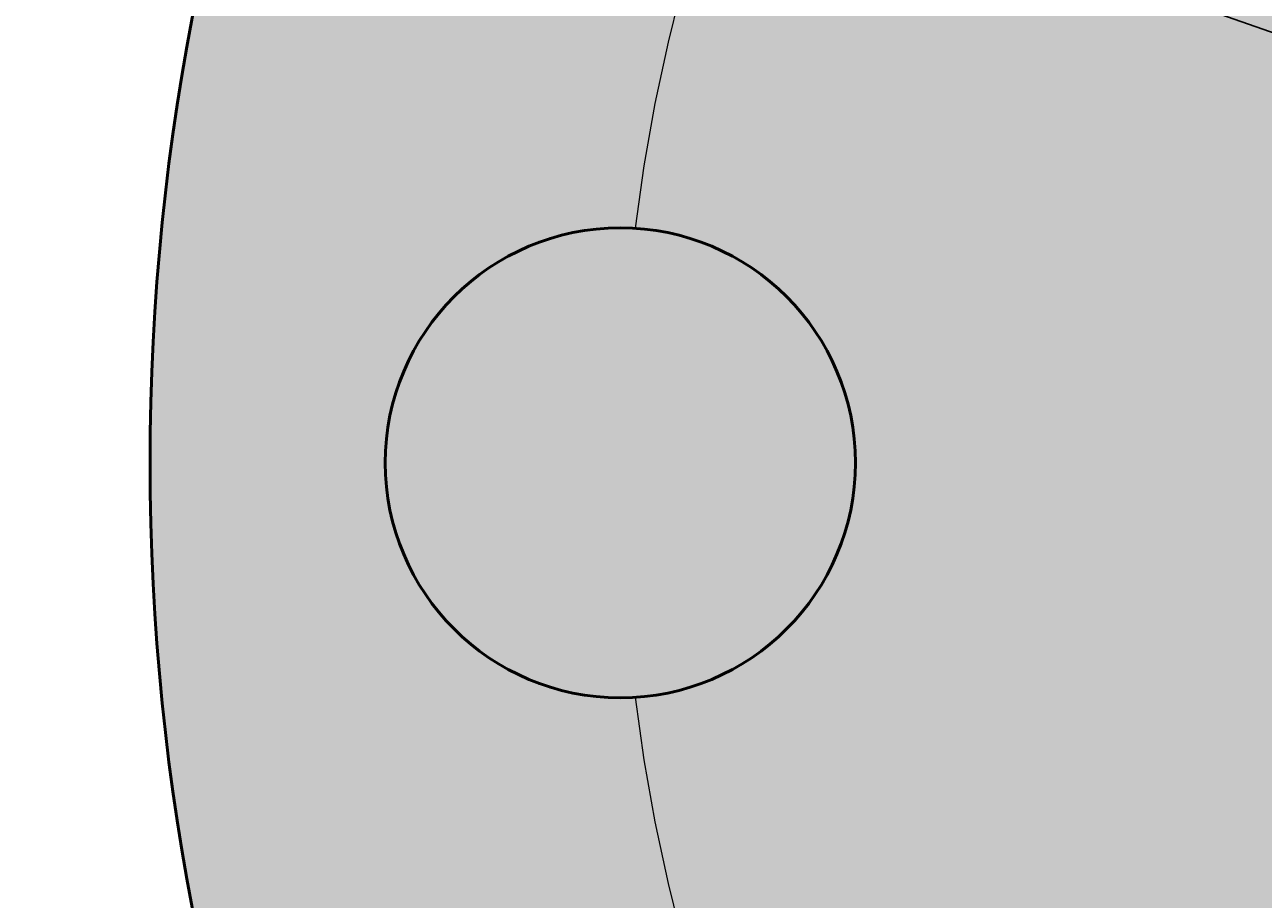
# Model space of a CAD drawing. Units: inches. Extents: x 139261 to 139415, y 52839 to 52963.
# Tile 4 of 20: x 139288 to 139314, y 52891 to 52910. Entities that reach past the tile are written whole.
import ezdxf

# ---------------------------------------------------------------- set-up
doc = ezdxf.new("R2010")
doc.units = ezdxf.units.IN
doc.header["$MEASUREMENT"] = 0
doc.linetypes.add('CENTER', pattern=[50.8, 31.75, -6.35, 6.35, -6.35])
for name, color, linetype, lineweight in [('M-CNTR', 4, 'CENTER', 18), ('M-DIMS', 2, 'Continuous', 25), ('M-HATC', 8, 'Continuous', 18), ('M-OUTL', 7, 'Continuous', 50)]:
    doc.layers.add(name, color=color, linetype=linetype, lineweight=lineweight)
doc.styles.get("Standard").update_dxf_attribs({"font": 'arial.ttf'})
doc.dimstyles.get("Standard").update_dxf_attribs({"dimtxt": 0.18, "dimasz": 0.18, "dimexe": 0.18, "dimexo": 0.0625, "dimgap": 0.09, "dimtad": 0, "dimtih": 1, "dimtoh": 1, "dimdec": 4, "dimzin": 0, "dimdsep": 46, "dimtxsty": 'Standard', "dimcen": 0.09, "dimadec": 0, "dimazin": 0, "dimtfac": 1, "dimtdec": 4, "dimtofl": 0, "dimtmove": 0, "dimatfit": 3, "dimfxl": 1, "dimtolj": 1, "dimtzin": 0, "dimarcsym": 0})

# ---------------------------------------------------------------- blocks, each defined once
blk = doc.blocks.new('*U1')
blk.add_circle((0, 0), 5)
blk = doc.blocks.new('*U2')
at = {"layer": 'M-OUTL', "color": 0, "linetype": 'ByBlock', "lineweight": -2, "transparency": 16777216, "rotation": 90}
blk.add_blockref('*U1', (139300.357, 52900.217), dxfattribs=at)
blk = doc.blocks.new('*D4')
at = {"layer": 'Defpoints', "color": 0, "transparency": 16777216}
for p in [(139373.053, 52923.26), (139307.661, 52877.175)]:
    blk.add_point(p, dxfattribs=at)
at = {"layer": 'M-DIMS', "color": 0, "lineweight": -2, "transparency": 16777216}
for p, q in [((139414.011, 52952.126), (139373.2, 52923.364)), ((139414.191, 52952.126), (139414.011, 52952.126)), ((139340.267, 52900.217), (139340.447, 52900.217)), ((139340.357, 52900.127), (139340.357, 52900.307))]:
    blk.add_line(p, q, dxfattribs=at)
blk.add_arc((139340.357, 52900.217), 40, 34.9168, 52.0771, dxfattribs=at)
at = {"layer": 'M-DIMS', "color": 0, "transparency": 16777216}
blk.add_solid([(139373.183, 52923.388), (139373.217, 52923.339), (139373.053, 52923.26)], dxfattribs=at)
at = {"layer": 'M-DIMS', "color": 0, "transparency": 16777216, "insert": (139414.822, 52952.126), "char_height": 0.18, "attachment_point": 5}
blk.add_mtext('\\A1;∅80.0000', dxfattribs=at)
blk = doc.blocks.new('*D5')
at = {"layer": 'Defpoints', "color": 0, "transparency": 16777216}
for p in [(139316.763, 52908.484), (139363.951, 52891.951)]:
    blk.add_point(p, dxfattribs=at)
at = {"layer": 'M-DIMS', "color": 0, "lineweight": -2, "transparency": 16777216}
for p, q in [((139262.553, 52927.414), (139262.733, 52927.414)), ((139262.733, 52927.414), (139316.593, 52908.544)), ((139340.267, 52900.217), (139340.447, 52900.217)), ((139340.357, 52900.127), (139340.357, 52900.307))]:
    blk.add_line(p, q, dxfattribs=at)
at = {"layer": 'M-DIMS', "color": 0, "transparency": 16777216}
blk.add_solid([(139316.603, 52908.572), (139316.583, 52908.515), (139316.763, 52908.484)], dxfattribs=at)
at = {"layer": 'M-DIMS', "color": 0, "transparency": 16777216, "insert": (139261.922, 52927.414), "char_height": 0.18, "attachment_point": 5}
blk.add_mtext('\\A1;∅50.0000', dxfattribs=at)
blk = doc.blocks.new('*D9')
at = {"layer": 'Defpoints', "color": 0, "transparency": 16777216}
for p in [(139302.054, 52932.357), (139378.659, 52868.078)]:
    blk.add_point(p, dxfattribs=at)
at = {"layer": 'M-DIMS', "color": 0, "lineweight": -2, "transparency": 16777216}
for p, q in [((139278.893, 52951.64), (139279.073, 52951.64)), ((139279.073, 52951.64), (139301.916, 52932.472)), ((139340.267, 52900.217), (139340.447, 52900.217)), ((139340.357, 52900.127), (139340.357, 52900.307))]:
    blk.add_line(p, q, dxfattribs=at)
at = {"layer": 'M-DIMS', "color": 0, "transparency": 16777216}
blk.add_solid([(139301.936, 52932.495), (139301.897, 52932.449), (139302.054, 52932.357)], dxfattribs=at)
at = {"layer": 'M-DIMS', "color": 0, "transparency": 16777216, "insert": (139278.506, 52951.64), "char_height": 0.18, "attachment_point": 5}
blk.add_mtext('\\A1;∅100', dxfattribs=at)

msp = doc.modelspace()

# ---------------------------------------------------------------- hatches: boundary and pattern name
at = {"layer": 'M-HATC'}
h = msp.add_hatch(color=256, dxfattribs=at)
h.dxf.hatch_style = 1
h.paths.add_polyline_path([(139290.35689, 52900.21749, 1), (139390.35689, 52900.21749, 1)])
h.paths.add_polyline_path([(139335.36666, 52939.90499, -0.01563646), (139335.35689, 52940.21749, -1), (139345.35689, 52940.21749, -0.01563646), (139345.34711, 52939.90499, -0.13461315), (139364.89157, 52931.80941, -0.691035), (139373.64116, 52928.50176, -0.21521822), (139371.94881, 52924.75216, -0.13461315), (139380.04439, 52905.20771, -0.43265224), (139385.35689, 52900.21749, -0.43265224), (139380.04439, 52895.22726, -0.13461315), (139371.94881, 52875.68281, -0.21521822), (139373.64116, 52871.93321, -0.691035), (139364.89157, 52868.62556, -0.13461315), (139345.34711, 52860.52999, -0.01563646), (139345.35689, 52860.21749, -1), (139335.35689, 52860.21749, -0.01563646), (139335.36666, 52860.52999, -0.13461315), (139315.82221, 52868.62556, -0.691035), (139307.07262, 52871.93321, -0.21521822), (139308.76496, 52875.68281, -0.13461315), (139300.66939, 52895.22726, -0.43265224), (139295.35689, 52900.21749, -0.43265224), (139300.66939, 52905.20771, -0.13461315), (139308.76496, 52924.75216, -0.21521822), (139307.07262, 52928.50176, -0.691035), (139315.82221, 52931.80941, -0.13461315)], flags=16)
h.paths.add_polyline_path([(139365.35689, 52900.21749, -1), (139315.35689, 52900.21749, -1)], flags=0)
h.paths.add_polyline_path([(139323.71474, 52911.30978), (139356.99903, 52911.30978, -0.3027197), (139356.99903, 52889.12519), (139323.71474, 52889.12519, -0.3027197)], flags=0)
h.paths.add_polyline_path([(139364.89157, 52931.80941, 0.13461315), (139345.34711, 52939.90499, -0.93933644), (139335.36666, 52939.90499, 0.13461315), (139315.82221, 52931.80941, -0.18270763), (139317.07262, 52928.50176, -0.64579494), (139308.76496, 52924.75216, 0.13461315), (139300.66939, 52905.20771, -0.39601219), (139305.35689, 52900.21749, -0.39601219), (139300.66939, 52895.22726, 0.13461315), (139308.76496, 52875.68281, -0.64579494), (139317.07262, 52871.93321, -0.18270763), (139315.82221, 52868.62556, 0.13461315), (139335.36666, 52860.52999, -0.93933644), (139345.34711, 52860.52999, 0.13461315), (139364.89157, 52868.62556, -0.18270763), (139363.64116, 52871.93321, -0.64579494), (139371.94881, 52875.68281, 0.13461315), (139380.04439, 52895.22726, -0.39601219), (139375.35689, 52900.21749, -0.39601219), (139380.04439, 52905.20771, 0.13461315), (139371.94881, 52924.75216, -0.64579494), (139363.64116, 52928.50176, -0.18270763)], flags=0)
h = msp.add_hatch(color=256, dxfattribs=at)
h.dxf.hatch_style = 1
h.set_gradient(color1=(205, 105, 40), tint=1)
h.paths.add_polyline_path([(139335.35689, 52940.21749, 1), (139345.35689, 52940.21749, 1)])
h.paths.add_polyline_path([(139307.07262, 52928.50176, 1), (139317.07262, 52928.50176, 1)])
h.paths.add_polyline_path([(139295.35689, 52900.21749, 1), (139305.35689, 52900.21749, 1)])
h.paths.add_polyline_path([(139307.07262, 52871.93321, 1), (139317.07262, 52871.93321, 1)])
h.paths.add_polyline_path([(139345.35689, 52860.21749, 1), (139335.35689, 52860.21749, 1)])
h.paths.add_polyline_path([(139363.64116, 52871.93321, 1), (139373.64116, 52871.93321, 1)])
h.paths.add_polyline_path([(139375.35689, 52900.21749, 1), (139385.35689, 52900.21749, 1)])
h.paths.add_polyline_path([(139363.64116, 52928.50176, 1), (139373.64116, 52928.50176, 1)])
h = msp.add_hatch(color=256, dxfattribs=at)
h.dxf.hatch_style = 1
h.paths.add_polyline_path([(139345.34711, 52939.90499, -0.93933644), (139335.36666, 52939.90499, 0.13461315), (139315.82221, 52931.80941, -0.18270763), (139317.07262, 52928.50176, -0.64579494), (139308.76496, 52924.75216, 0.13461315), (139300.66939, 52905.20771, -0.39601219), (139305.35689, 52900.21749, -0.39601219), (139300.66939, 52895.22726, 0.13461315), (139308.76496, 52875.68281, -0.64579494), (139317.07262, 52871.93321, -0.18270763), (139315.82221, 52868.62556, 0.13461315), (139335.36666, 52860.52999, -0.93933644), (139345.34711, 52860.52999, 0.13461315), (139364.89157, 52868.62556, -0.18270763), (139363.64116, 52871.93321, -0.64579494), (139371.94881, 52875.68281, 0.13461315), (139380.04439, 52895.22726, -0.39601219), (139375.35689, 52900.21749, -0.39601219), (139380.04439, 52905.20771, 0.13461315), (139371.94881, 52924.75216, -0.64579494), (139363.64116, 52928.50176, -0.18270763), (139364.89157, 52931.80941, 0.13461315)])
h.paths.add_polyline_path([(139365.35689, 52900.21749, -1), (139315.35689, 52900.21749, -1)], flags=16)
h.paths.add_polyline_path([(139356.99903, 52911.30978, -0.3027197), (139356.99903, 52889.12519), (139323.71474, 52889.12519, -0.3027197), (139323.71474, 52911.30978)], flags=0)

# ---------------------------------------------------------------- linework, layer by layer
at = {"layer": 'M-CNTR'}
for start, end in [(142.166643, 172.833357), (187.166643, 217.833357)]:
    msp.add_arc((139340.35689, 52900.21749), 40, start, end, dxfattribs=at)
at = {"layer": 'M-OUTL'}
msp.add_circle((139340.35689, 52900.21749), 50, dxfattribs=at)

# ---------------------------------------------------------------- block references
msp.add_blockref('*U2', (0, 0), dxfattribs=at)

# ---------------------------------------------------------------- dimensions: what is measured, and where the dimension line sits
at = {"layer": 'M-DIMS'}
for p1, p2, override, picture, middle in [((139307.66087, 52877.17469), (139373.0529, 52923.26028), {"dimclrd": 0, "dimclre": 0, "dimclrt": 0}, '*D4', (139414.82217, 52952.12585)), ((139378.65939, 52868.07845), (139302.05438, 52932.35652), {"dimdec": 0, "dimlfac": 1, "dimrnd": 0, "dimzin": 0, "dimdsep": 46, "dimlunit": 2}, '*D9', (139278.50641, 52951.63995)), ((139363.95063, 52891.95098), (139316.76314, 52908.48399), {"dimclrd": 0, "dimclre": 0, "dimclrt": 0}, '*D5', (139261.92224, 52927.41429))]:
    dim = msp.add_diameter_dim_2p(p1=p1, p2=p2, dimstyle='Standard', override=override, dxfattribs=at)
    dim.commit()
    dim.dimension.update_dxf_attribs({"geometry": picture, "text_midpoint": middle, "dimtype": 163})

doc.saveas('drawing.dxf')
